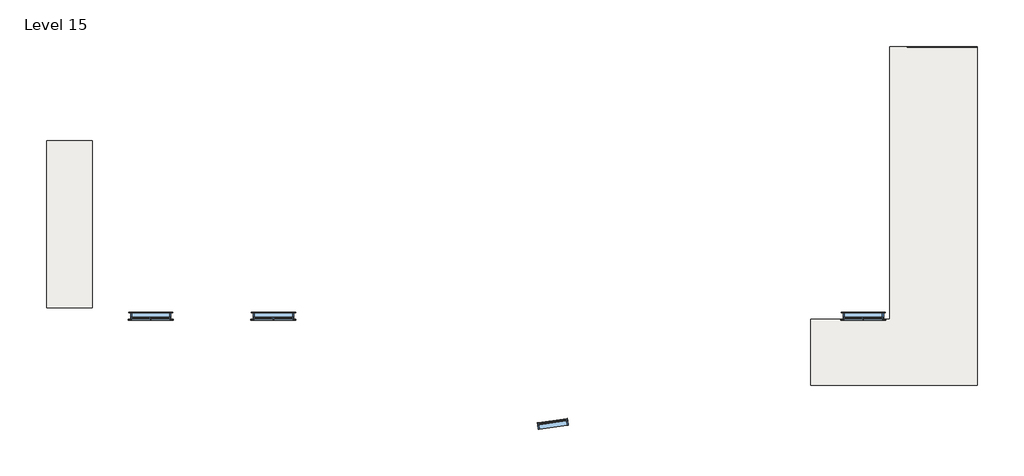
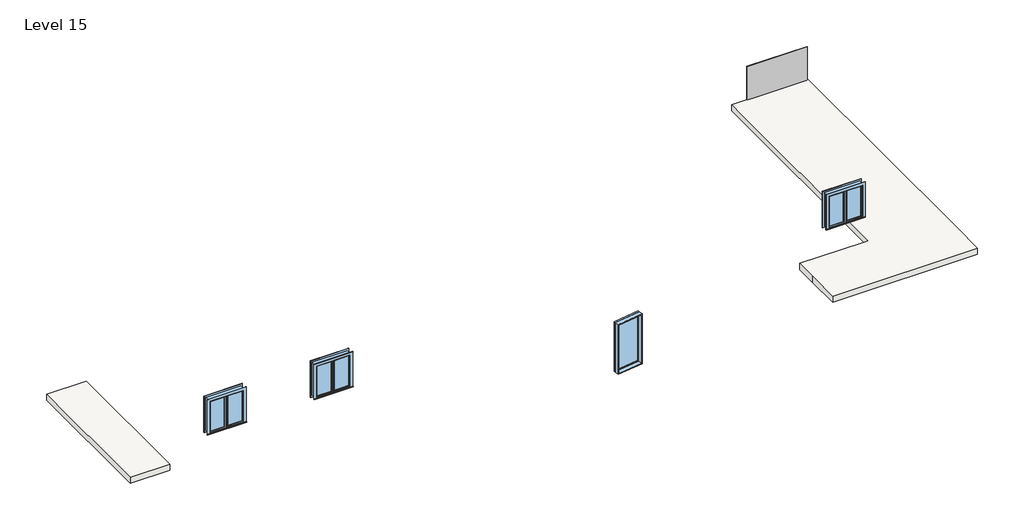
# One storey: 4 windows, 2 slabs, 1 plate.
"""IFC4 building model written with IfcOpenShell, lengths in millimetres."""

from ifc_helpers import new_model, si_unit, frame, origin, place, context, project, spatial, polyline, outline, extrude, transform, mapped, element, save
from components import system_panel_glazed_4fcd3a06, window_0862ab64, window_9a779fa2

model = new_model("IFC4")

# Units and contexts
model_context = context("Model", 3, world=origin())
ifc_project = project(units=[si_unit("LENGTHUNIT", "METRE", prefix="MILLI")], contexts=[model_context])

# Site, building, storey
site = spatial("IfcSite", under=ifc_project)
building = spatial("IfcBuilding", under=site)
storey = spatial("IfcBuildingStorey", under=building, Name="Level 15", Elevation=22936.2)

# Plate
placement = place(None, origin())
system_panel_glazed_shape = system_panel_glazed_4fcd3a06(model_context)
element("IfcPlate", 1, ObjectType="System Panel : Glazed", at=placement, inside=storey, context=model_context, shape_type="MappedRepresentation", body=[
    mapped(system_panel_glazed_shape, transform((9031.7964352, -5892.9308221, 22936.2), x_axis=(1.0, 0.0, 0.0), y_axis=(0.0, 1.0, 0.0), z_axis=(0.0, 0.0, 1.0))),
])

# Slabs
element("IfcSlab", 2, ObjectType="9\"", at=placement, inside=storey, context=model_context, shape_type="SweptSolid", body=[
    extrude(outline(polyline([(-17972.8272291, -8690.0239591), (-16601.2272291, -8690.0239591), (-16601.2272291, -13719.2239591), (-17972.8272291, -13719.2239591), (-17972.8272291, -8690.0239591)])), frame((0.0, 0.0, 22707.6), z_axis=(0.0, 0.0, 1.0), x_axis=(1.0, 0.0, 0.0)), (0.0, 0.0, 1.0), 228.6),
])
element("IfcSlab", 3, ObjectType="9\"", at=placement, inside=storey, context=model_context, shape_type="SweptSolid", body=[
    extrude(outline(polyline([(5071.9618272, -14840.0808221), (5071.9618272, -14078.0808221), (7256.3618272, -14078.0808221), (7459.5618272, -14078.0808221), (7459.5618272, -5848.4808221), (10101.1618272, -5848.4808221), (10101.1618272, -14840.0808221), (10101.1618272, -16059.2808221), (5071.9618272, -16059.2808221), (5071.9618272, -14840.0808221)])), frame((0.0, 0.0, 22707.6), z_axis=(0.0, 0.0, 1.0), x_axis=(1.0, 0.0, 0.0)), (0.0, 0.0, 1.0), 228.6),
])

# Windows
window_shape = window_0862ab64(model_context)
element("IfcWindow", 4, ObjectType="Casement Dbl with Trim : 48\" x 48\"", at=placement, inside=storey, context=model_context, shape_type="MappedRepresentation", body=[
    mapped(window_shape, transform((-14829.9505427, -13957.4308221, 22936.2), x_axis=(-1.0, 0.0, 0.0), y_axis=(0.0, -1.0, 0.0), z_axis=(0.0, 0.0, 1.0))),
])
element("IfcWindow", 5, ObjectType="Casement Dbl with Trim : 48\" x 48\"", at=placement, inside=storey, context=model_context, shape_type="MappedRepresentation", body=[
    mapped(window_shape, transform((-11129.6382271, -13957.4308221, 22936.2), x_axis=(-1.0, 0.0, 0.0), y_axis=(0.0, -1.0, 0.0), z_axis=(0.0, 0.0, 1.0))),
])
element("IfcWindow", 6, ObjectType="Casement Dbl with Trim : 48\" x 48\"", at=placement, inside=storey, context=model_context, shape_type="MappedRepresentation", body=[
    mapped(window_shape, transform((6658.4494573, -13957.4308221, 22936.2), x_axis=(-1.0, 0.0, 0.0), y_axis=(0.0, -1.0, 0.0), z_axis=(0.0, 0.0, 1.0))),
])
window_2_shape = window_9a779fa2(model_context)
element("IfcWindow", 7, ObjectType="Fixed : 36\" x 72\"", at=placement, inside=storey, context=model_context, shape_type="MappedRepresentation", body=[
    mapped(window_2_shape, transform((-2665.8073792, -17224.4013647, 23438.6621165), x_axis=(0.9900693758779321, 0.14057962494146128, 0.0), y_axis=(-0.14057962494146128, 0.9900693758779321, 0.0), z_axis=(0.0, 0.0, 1.0))),
])

save(model, "model.ifc")

# Revit data of these elements
# Type "System Panel : Glazed"
#   Construction Type Id = "GSP4R"
#   Analytic Construction = "1/8 in Pilkington single glazing"
#   Visual Light Transmittance = 0.9
#   Solar Heat Gain Coefficient = 0.86
#   Heat Transfer Coefficient (U) = 1.18115 BTU/(h·ft²·°F)
# Type "9\""
#   Assembly Code = "B1010"
#   Function = 0
#   Layers, outside or top first: 0' - 9" no material (function 1)
# Type "Casement Dbl with Trim : 48\" x 48\""
#   Type Mark = "10"
#   Construction Type Id = "GSP4R"
#   Assembly Code = "B2020100"
#   Analytic Construction = "1/8 in Pilkington single glazing"
#   Visual Light Transmittance = 0.9
#   Solar Heat Gain Coefficient = 0.78
#   Heat Transfer Coefficient (U) = 0.6496 BTU/(h·ft²·°F)
#   Height = 4' - 0"
#   Default Sill Height = 3' - 0"
#   Trim Projection - Ext. = 0' - 0 1/2"
#   Trim Projection - Int. = 0' - 0 3/4"
#   Trim Width - Exterior = 0' - 3 1/2"
#   Trim Width - Interior = 0' - 3 1/2"
#   Width = 4' - 0"
#   Window Inset = 0' - 0 3/4"
#   Define Thermal Properties by = 1
#   Glass Pane Material = Glass
#   Sash Material = Sash
#   Trim Exterior Material = Trim
#   Trim Interior Material = Trim
#   Wall Closure = (empty or 0)
# Type "Fixed : 36\" x 72\""
#   Type Mark = "9"
#   Construction Type Id = "GSP4R"
#   Assembly Code = "B2020100"
#   Analytic Construction = "1/8 in Pilkington single glazing"
#   Visual Light Transmittance = 0.9
#   Solar Heat Gain Coefficient = 0.78
#   Heat Transfer Coefficient (U) = 0.6496 BTU/(h·ft²·°F)
#   Height = 6' - 0"
#   Default Sill Height = 1' - 0"
#   Width = 3' - 0"
#   Window Inset = 0' - 0 3/4"
#   Define Thermal Properties by = 1
#   Glass Pane Material = Glass
#   Sash Material = Sash
#   Wall Closure = (empty or 0)
# Element 1 (IfcPlate, "System Panel : Glazed")
#   Phase Created = New Construction
#   Materials on its faces: "Glass"
# Element 2 (IfcSlab, "9\"")
#   built-in parameter 1001955 = 3.14159 (stored number, unit not read)
#   Height Offset From Level = 0' - 0"
#   Phase Created = New Construction
#   Materials on its faces: "Default Floor"
# Element 3 (IfcSlab, "9\"")
#   built-in parameter 1001955 = -1.5708 (stored number, unit not read)
#   Height Offset From Level = 0' - 0"
#   Phase Created = New Construction
#   Materials on its faces: "Default Floor"
# Element 4 (IfcWindow, "Casement Dbl with Trim : 48\" x 48\"")
#   Mark = "33"
#   Phase Created = New Construction
#   Materials on its faces: "Sash", "Trim", "Glass"
# Element 5 (IfcWindow, "Casement Dbl with Trim : 48\" x 48\"")
#   Mark = "34"
#   Phase Created = New Construction
#   Materials on its faces: "Sash", "Trim", "Glass"
# Element 6 (IfcWindow, "Casement Dbl with Trim : 48\" x 48\"")
#   Mark = "54"
#   Phase Created = New Construction
#   Materials on its faces: "Sash", "Trim", "Glass"
# Element 7 (IfcWindow, "Fixed : 36\" x 72\"")
#   Mark = "9"
#   Phase Created = New Construction
#   Materials on its faces: "Sash", "Glass"
# Materials
#   "Glass": class "Glass", colour RGB 0 128 192, transparency 0.75, Description = "Soda Lime Glass", Cost = 0
#   "Sash": class "Wood", colour RGB 224 178 126, transparency 0
#   "Trim": class "Wood", colour RGB 224 178 126, transparency 0
#   "Default Floor": colour RGB 128 128 128, transparency 0
